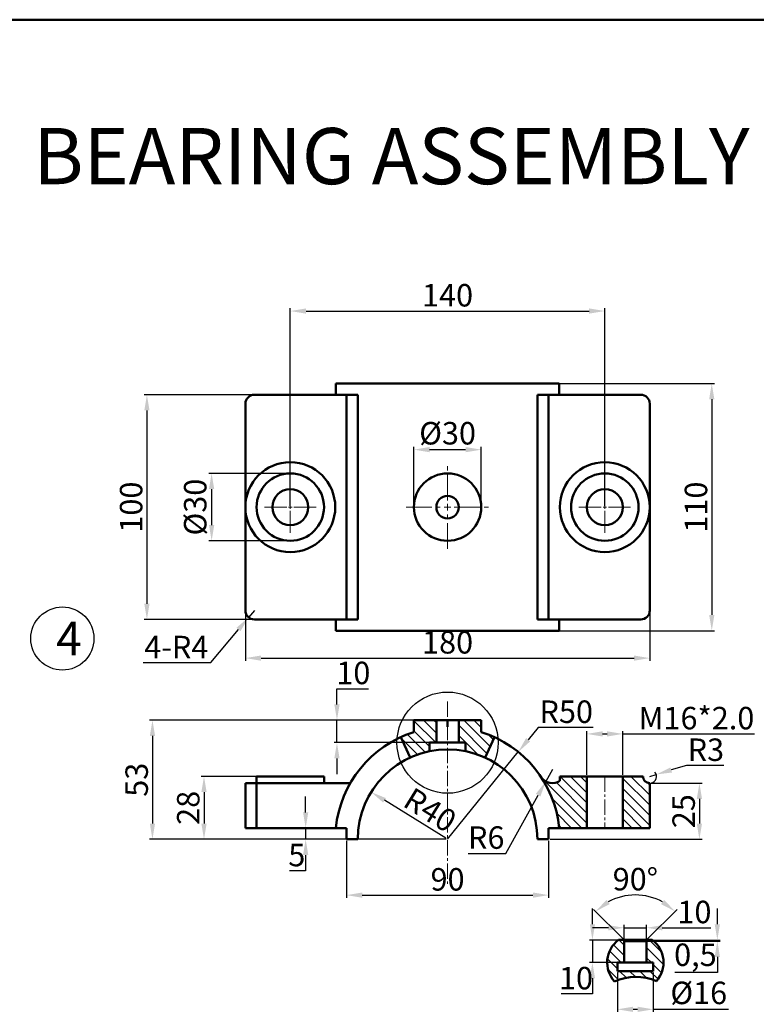
# Model space of a CAD drawing. Units: millimetres. Extents: x -68 to 1086, y -293 to 557.
# Tile 3 of 4: x 373 to 701, y 119 to 557. Entities that reach past the tile are written whole.
import ezdxf

# ---------------------------------------------------------------- set-up
doc = ezdxf.new("R2010")
doc.units = ezdxf.units.MM
doc.header["$LTSCALE"] = 0.6
doc.linetypes.add('CENTER2', pattern=[28.575, 19.05, -3.175, 3.175, -3.175])
for name, color, linetype, lineweight in [('M-CNTR', 1, 'CENTER2', 18), ('M-DIMS', 2, 'Continuous', 25), ('M-HATC', 8, 'Continuous', 18), ('M-OUTL', 7, 'Continuous', 50), ('M-SYMB', 4, 'Continuous', 25), ('M-TEXT', 3, 'Continuous', 25)]:
    doc.layers.add(name, color=color, linetype=linetype, lineweight=lineweight)
doc.styles.get("Standard").update_dxf_attribs({"font": 'arial.ttf'})
doc.dimstyles.new('ISO-25', dxfattribs={"dimtxt": 10, "dimasz": 7, "dimexe": 1.25, "dimexo": 0.625, "dimtad": 1, "dimtoh": 1, "dimtxsty": 'Standard', "dimcen": 2.5, "dimadec": 0, "dimazin": 0, "dimtfac": 1, "dimtmove": 0, "dimatfit": 3, "dimfxl": 1, "dimarcsym": 0})
pattern_1 = [(135, (-319.924, -184.7082), (-2.245064, -2.245064), [])]

# ---------------------------------------------------------------- blocks, each defined once
blk = doc.blocks.new('*U22')
at = {"layer": 'M-CNTR', "color": 0, "transparency": 16777216}
for p, q in [((0, 1.6), (0, 11.5)), ((-11.5, 0), (-1.6, 0)), ((1.6, 0), (11.5, 0)), ((0, -11.5), (0, -1.6))]:
    blk.add_line(p, q, dxfattribs=at)
at = {"layer": 'M-CNTR', "color": 0, "linetype": 'Continuous', "transparency": 16777216}
for p, q in [((-0.8, 0), (0.8, 0)), ((0, -0.8), (0, 0.8))]:
    blk.add_line(p, q, dxfattribs=at)
blk = doc.blocks.new('*U23')
at = {"layer": 'M-CNTR', "color": 0, "transparency": 16777216}
for p, q in [((0, 1.6), (0, 11.5)), ((-11.5, 0), (-1.6, 0)), ((1.6, 0), (11.5, 0)), ((0, -11.5), (0, -1.6))]:
    blk.add_line(p, q, dxfattribs=at)
at = {"layer": 'M-CNTR', "color": 0, "linetype": 'Continuous', "transparency": 16777216}
for p, q in [((-0.8, 0), (0.8, 0)), ((0, -0.8), (0, 0.8))]:
    blk.add_line(p, q, dxfattribs=at)
blk = doc.blocks.new('*U24')
at = {"layer": 'M-CNTR', "color": 0, "transparency": 16777216}
for p, q in [((0, 3), (0, 18.5)), ((-18.5, 0), (-3, 0)), ((3, 0), (18.5, 0)), ((0, -18.5), (0, -3))]:
    blk.add_line(p, q, dxfattribs=at)
at = {"layer": 'M-CNTR', "color": 0, "linetype": 'Continuous', "transparency": 16777216}
for p, q in [((-1.5, 0), (1.5, 0)), ((0, -1.5), (0, 1.5))]:
    blk.add_line(p, q, dxfattribs=at)
blk = doc.blocks.new('*D25')
at = {"layer": 'Defpoints', "color": 0, "ltscale": 0.6, "transparency": 16777216}
for p in [(563.31, 244.93), (431.94, 191.93), (563.31, 191.93)]:
    blk.add_point(p, dxfattribs=at)
at = {"layer": 'M-DIMS', "color": 0, "lineweight": -2, "ltscale": 0.6, "transparency": 16777216}
for p, q in [((562.68, 244.93), (430.69, 244.93)), ((431.94, 237.93), (431.94, 198.93)), ((562.68, 191.93), (430.69, 191.93))]:
    blk.add_line(p, q, dxfattribs=at)
at = {"layer": 'M-DIMS', "color": 0, "ltscale": 0.6, "transparency": 16777216}
for points in [[(430.78, 237.93), (433.11, 237.93), (431.94, 244.93)], [(430.78, 198.93), (433.11, 198.93), (431.94, 191.93)]]:
    blk.add_solid(points, dxfattribs=at)
at = {"layer": 'M-DIMS', "color": 0, "ltscale": 0.6, "transparency": 16777216, "insert": (426.21, 218.43), "char_height": 10, "attachment_point": 5, "rotation": 90}
blk.add_mtext('53', dxfattribs=at)
blk = doc.blocks.new('*D26')
at = {"layer": 'Defpoints', "color": 0, "ltscale": 0.6, "transparency": 16777216}
for p in [(493.31, 219.93), (454.89, 191.93), (493.31, 191.93)]:
    blk.add_point(p, dxfattribs=at)
at = {"layer": 'M-DIMS', "color": 0, "lineweight": -2, "ltscale": 0.6, "transparency": 16777216}
for p, q in [((492.68, 219.93), (453.64, 219.93)), ((454.89, 212.93), (454.89, 198.93)), ((492.68, 191.93), (453.64, 191.93))]:
    blk.add_line(p, q, dxfattribs=at)
at = {"layer": 'M-DIMS', "color": 0, "ltscale": 0.6, "transparency": 16777216}
for points in [[(453.72, 212.93), (456.05, 212.93), (454.89, 219.93)], [(453.72, 198.93), (456.05, 198.93), (454.89, 191.93)]]:
    blk.add_solid(points, dxfattribs=at)
at = {"layer": 'M-DIMS', "color": 0, "ltscale": 0.6, "transparency": 16777216, "insert": (449.16, 205.93), "char_height": 10, "attachment_point": 5, "rotation": 90}
blk.add_mtext('28', dxfattribs=at)
blk = doc.blocks.new('*D27')
at = {"layer": 'Defpoints', "color": 0, "ltscale": 0.6, "transparency": 16777216}
for p in [(563.31, 244.93), (514.07, 234.93), (563.31, 234.93)]:
    blk.add_point(p, dxfattribs=at)
at = {"layer": 'M-DIMS', "color": 0, "lineweight": -2, "ltscale": 0.6, "transparency": 16777216}
for p, q in [((514.07, 251.93), (514.07, 258.93)), ((514.07, 258.93), (528.04, 258.93)), ((562.68, 244.93), (512.82, 244.93)), ((514.07, 234.93), (514.07, 244.93)), ((562.68, 234.93), (512.82, 234.93)), ((514.07, 227.93), (514.07, 220.93))]:
    blk.add_line(p, q, dxfattribs=at)
at = {"layer": 'M-DIMS', "color": 0, "ltscale": 0.6, "transparency": 16777216}
for points in [[(512.9, 251.93), (515.24, 251.93), (514.07, 244.93)], [(512.9, 227.93), (515.24, 227.93), (514.07, 234.93)]]:
    blk.add_solid(points, dxfattribs=at)
at = {"layer": 'M-DIMS', "color": 0, "ltscale": 0.6, "transparency": 16777216, "insert": (521.37, 264.66), "char_height": 10, "attachment_point": 5}
blk.add_mtext('10', dxfattribs=at)
blk = doc.blocks.new('*D28')
at = {"layer": 'Defpoints', "color": 0, "ltscale": 0.6, "transparency": 16777216}
for p in [(653.31, 216.93), (608.31, 191.93), (675.42, 191.93)]:
    blk.add_point(p, dxfattribs=at)
at = {"layer": 'M-DIMS', "color": 0, "lineweight": -2, "ltscale": 0.6, "transparency": 16777216}
for p, q in [((653.93, 216.93), (676.67, 216.93)), ((675.42, 209.93), (675.42, 198.93)), ((608.93, 191.93), (676.67, 191.93))]:
    blk.add_line(p, q, dxfattribs=at)
at = {"layer": 'M-DIMS', "color": 0, "ltscale": 0.6, "transparency": 16777216}
for points in [[(674.25, 209.93), (676.58, 209.93), (675.42, 216.93)], [(674.25, 198.93), (676.58, 198.93), (675.42, 191.93)]]:
    blk.add_solid(points, dxfattribs=at)
at = {"layer": 'M-DIMS', "color": 0, "ltscale": 0.6, "transparency": 16777216, "insert": (669.69, 204.43), "char_height": 10, "attachment_point": 5, "rotation": 90}
blk.add_mtext('25', dxfattribs=at)
blk = doc.blocks.new('*D29')
at = {"layer": 'Defpoints', "color": 0, "ltscale": 0.6, "transparency": 16777216}
for p in [(518.31, 191.93), (608.31, 191.93), (608.31, 167.1)]:
    blk.add_point(p, dxfattribs=at)
at = {"layer": 'M-DIMS', "color": 0, "lineweight": -2, "ltscale": 0.6, "transparency": 16777216}
for p, q in [((518.31, 191.31), (518.31, 165.85)), ((608.31, 191.31), (608.31, 165.85)), ((525.31, 167.1), (601.31, 167.1))]:
    blk.add_line(p, q, dxfattribs=at)
at = {"layer": 'M-DIMS', "color": 0, "ltscale": 0.6, "transparency": 16777216}
for points in [[(525.31, 168.26), (525.31, 165.93), (518.31, 167.1)], [(601.31, 168.26), (601.31, 165.93), (608.31, 167.1)]]:
    blk.add_solid(points, dxfattribs=at)
at = {"layer": 'M-DIMS', "color": 0, "ltscale": 0.6, "transparency": 16777216, "insert": (563.31, 172.83), "char_height": 10, "attachment_point": 5}
blk.add_mtext('90', dxfattribs=at)
blk = doc.blocks.new('*D30')
at = {"layer": 'Defpoints', "color": 0, "ltscale": 0.6, "transparency": 16777216}
for p in [(529.28, 212.96), (563.31, 191.93)]:
    blk.add_point(p, dxfattribs=at)
at = {"layer": 'M-DIMS', "color": 0, "lineweight": -2, "ltscale": 0.6, "transparency": 16777216}
blk.add_line((562.55, 192.4), (535.24, 209.28), dxfattribs=at)
at = {"layer": 'M-DIMS', "color": 0, "ltscale": 0.6, "transparency": 16777216}
blk.add_solid([(535.85, 210.27), (534.63, 208.29), (529.28, 212.96)], dxfattribs=at)
at = {"layer": 'M-DIMS', "color": 0, "ltscale": 0.6, "transparency": 16777216, "insert": (554.89, 203.88), "char_height": 10, "attachment_point": 5, "rotation": 328.282}
blk.add_mtext('R40', dxfattribs=at)
blk = doc.blocks.new('*D31')
at = {"layer": 'Defpoints', "color": 0, "ltscale": 0.6, "transparency": 16777216}
for p in [(594.77, 230.8), (563.31, 191.93)]:
    blk.add_point(p, dxfattribs=at)
at = {"layer": 'M-DIMS', "color": 0, "lineweight": -2, "ltscale": 0.6, "transparency": 16777216}
for p, q in [((603.58, 241.68), (599.17, 236.24)), ((628.06, 241.68), (603.58, 241.68)), ((563.31, 191.93), (594.77, 230.8))]:
    blk.add_line(p, q, dxfattribs=at)
at = {"layer": 'M-DIMS', "color": 0, "ltscale": 0.6, "transparency": 16777216}
blk.add_solid([(598.26, 236.97), (600.08, 235.5), (594.77, 230.8)], dxfattribs=at)
at = {"layer": 'M-DIMS', "color": 0, "ltscale": 0.6, "transparency": 16777216, "insert": (616.13, 247.41), "char_height": 10, "attachment_point": 5}
blk.add_mtext('R50', dxfattribs=at)
blk = doc.blocks.new('*D32')
at = {"layer": 'Defpoints', "color": 0, "ltscale": 0.6, "transparency": 16777216}
for p in [(609.95, 222.93), (607.03, 217.69)]:
    blk.add_point(p, dxfattribs=at)
at = {"layer": 'M-DIMS', "color": 0, "lineweight": -2, "ltscale": 0.6, "transparency": 16777216}
for p, q in [((609.95, 222.93), (607.03, 217.69)), ((589.2, 185.68), (603.62, 211.57)), ((572.46, 185.68), (589.2, 185.68))]:
    blk.add_line(p, q, dxfattribs=at)
at = {"layer": 'M-DIMS', "color": 0, "ltscale": 0.6, "transparency": 16777216}
blk.add_solid([(602.6, 212.14), (604.64, 211.01), (607.03, 217.69)], dxfattribs=at)
at = {"layer": 'M-DIMS', "color": 0, "ltscale": 0.6, "transparency": 16777216, "insert": (580.52, 191.41), "char_height": 10, "attachment_point": 5}
blk.add_mtext('R6', dxfattribs=at)
blk = doc.blocks.new('*D33')
at = {"layer": 'Defpoints', "color": 0, "ltscale": 0.6, "transparency": 16777216}
for p in [(518.31, 196.93), (500.14, 191.93), (518.31, 191.93)]:
    blk.add_point(p, dxfattribs=at)
at = {"layer": 'M-DIMS', "color": 0, "lineweight": -2, "ltscale": 0.6, "transparency": 16777216}
for p, q in [((500.14, 203.93), (500.14, 210.93)), ((517.68, 196.93), (498.89, 196.93)), ((500.14, 196.93), (500.14, 191.93)), ((517.68, 191.93), (498.89, 191.93)), ((500.14, 184.93), (500.14, 177.93)), ((500.14, 177.93), (492.88, 177.93))]:
    blk.add_line(p, q, dxfattribs=at)
at = {"layer": 'M-DIMS', "color": 0, "ltscale": 0.6, "transparency": 16777216}
for points in [[(498.97, 203.93), (501.3, 203.93), (500.14, 196.93)], [(498.97, 184.93), (501.3, 184.93), (500.14, 191.93)]]:
    blk.add_solid(points, dxfattribs=at)
at = {"layer": 'M-DIMS', "color": 0, "ltscale": 0.6, "transparency": 16777216, "insert": (496.2, 183.64), "char_height": 10, "attachment_point": 5}
blk.add_mtext('5', dxfattribs=at)
blk = doc.blocks.new('*D34')
at = {"layer": 'Defpoints', "color": 0, "ltscale": 0.6, "transparency": 16777216}
for p in [(638.9, 133.33), (654.9, 133.33), (654.9, 116.29)]:
    blk.add_point(p, dxfattribs=at)
at = {"layer": 'M-DIMS', "color": 0, "lineweight": -2, "ltscale": 0.6, "transparency": 16777216}
for p, q in [((638.9, 132.7), (638.9, 115.04)), ((654.9, 132.7), (654.9, 115.04)), ((645.9, 116.29), (647.9, 116.29)), ((654.9, 116.29), (688.35, 116.29))]:
    blk.add_line(p, q, dxfattribs=at)
at = {"layer": 'M-DIMS', "color": 0, "ltscale": 0.6, "transparency": 16777216}
for points in [[(645.9, 117.46), (645.9, 115.12), (638.9, 116.29)], [(647.9, 117.46), (647.9, 115.12), (654.9, 116.29)]]:
    blk.add_solid(points, dxfattribs=at)
at = {"layer": 'M-DIMS', "color": 0, "ltscale": 0.6, "transparency": 16777216, "insert": (675.12, 122.3), "char_height": 10, "attachment_point": 5}
blk.add_mtext('%%C16', dxfattribs=at)
blk = doc.blocks.new('*D35')
at = {"layer": 'Defpoints', "color": 0, "ltscale": 0.6, "transparency": 16777216}
for p in [(641.9, 147.13), (627.79, 137.13), (641.9, 137.13)]:
    blk.add_point(p, dxfattribs=at)
at = {"layer": 'M-DIMS', "color": 0, "lineweight": -2, "ltscale": 0.6, "transparency": 16777216}
for p, q in [((627.79, 154.13), (627.79, 161.13)), ((641.28, 147.13), (626.54, 147.13)), ((627.79, 147.13), (627.79, 137.13)), ((641.28, 137.13), (626.54, 137.13)), ((627.79, 130.13), (627.79, 123.13)), ((627.79, 123.13), (613.82, 123.13))]:
    blk.add_line(p, q, dxfattribs=at)
at = {"layer": 'M-DIMS', "color": 0, "ltscale": 0.6, "transparency": 16777216}
for points in [[(626.63, 154.13), (628.96, 154.13), (627.79, 147.13)], [(626.63, 130.13), (628.96, 130.13), (627.79, 137.13)]]:
    blk.add_solid(points, dxfattribs=at)
at = {"layer": 'M-DIMS', "color": 0, "ltscale": 0.6, "transparency": 16777216, "insert": (620.49, 128.87), "char_height": 10, "attachment_point": 5}
blk.add_mtext('10', dxfattribs=at)
blk = doc.blocks.new('*D36')
at = {"layer": 'Defpoints', "color": 0, "ltscale": 0.6, "transparency": 16777216}
for p in [(653.38, 166.33), (641.9, 147.13), (642.4, 146.63), (651.4, 146.63), (651.9, 147.13)]:
    blk.add_point(p, dxfattribs=at)
at = {"layer": 'M-DIMS', "color": 0, "lineweight": -2, "ltscale": 0.6, "transparency": 16777216}
for p, q in [((641.46, 147.58), (628.31, 160.73)), ((652.34, 147.58), (665.49, 160.73))]:
    blk.add_line(p, q, dxfattribs=at)
blk.add_arc((646.9, 142.13), 25.05, 61.0658, 118.9342, dxfattribs=at)
at = {"layer": 'M-DIMS', "color": 0, "ltscale": 0.6, "transparency": 16777216}
for points in [[(635.48, 163.12), (634.08, 164.99), (629.19, 159.85)], [(659.72, 164.99), (658.32, 163.12), (664.61, 159.85)]]:
    blk.add_solid(points, dxfattribs=at)
at = {"layer": 'M-DIMS', "color": 0, "ltscale": 0.6, "transparency": 16777216, "insert": (646.9, 172.91), "char_height": 10, "attachment_point": 5}
blk.add_mtext('90°', dxfattribs=at)
blk = doc.blocks.new('*D37')
at = {"layer": 'Defpoints', "color": 0, "ltscale": 0.6, "transparency": 16777216}
for p in [(651.9, 152.57), (641.9, 147.13), (651.9, 147.13)]:
    blk.add_point(p, dxfattribs=at)
at = {"layer": 'M-DIMS', "color": 0, "lineweight": -2, "ltscale": 0.6, "transparency": 16777216}
for p, q in [((641.9, 147.76), (641.9, 153.82)), ((651.9, 147.76), (651.9, 153.82)), ((634.9, 152.57), (627.9, 152.57)), ((641.9, 152.57), (651.9, 152.57)), ((658.9, 152.57), (680.5, 152.57))]:
    blk.add_line(p, q, dxfattribs=at)
at = {"layer": 'M-DIMS', "color": 0, "ltscale": 0.6, "transparency": 16777216}
for points in [[(634.9, 153.74), (634.9, 151.41), (641.9, 152.57)], [(658.9, 153.74), (658.9, 151.41), (651.9, 152.57)]]:
    blk.add_solid(points, dxfattribs=at)
at = {"layer": 'M-DIMS', "color": 0, "ltscale": 0.6, "transparency": 16777216, "insert": (673.2, 158.3), "char_height": 10, "attachment_point": 5}
blk.add_mtext('10', dxfattribs=at)
blk = doc.blocks.new('*D38')
at = {"layer": 'Defpoints', "color": 0, "ltscale": 0.6, "transparency": 16777216}
for p in [(651.29, 147.13), (651.29, 146.63), (683.4, 146.63)]:
    blk.add_point(p, dxfattribs=at)
at = {"layer": 'M-DIMS', "color": 0, "lineweight": -2, "ltscale": 0.6, "transparency": 16777216}
for p, q in [((683.4, 154.13), (683.4, 161.13)), ((651.92, 147.13), (684.65, 147.13)), ((651.92, 146.63), (684.65, 146.63)), ((683.4, 147.13), (683.4, 146.63)), ((683.4, 139.63), (683.4, 132.63)), ((683.4, 132.63), (664.49, 132.63))]:
    blk.add_line(p, q, dxfattribs=at)
at = {"layer": 'M-DIMS', "color": 0, "ltscale": 0.6, "transparency": 16777216}
for points in [[(682.23, 154.13), (684.57, 154.13), (683.4, 147.13)], [(682.23, 139.63), (684.57, 139.63), (683.4, 146.63)]]:
    blk.add_solid(points, dxfattribs=at)
at = {"layer": 'M-DIMS', "color": 0, "ltscale": 0.6, "transparency": 16777216, "insert": (673.63, 139.27), "char_height": 10, "attachment_point": 5}
blk.add_mtext('0,5', dxfattribs=at)
blk = doc.blocks.new('*D39')
at = {"layer": 'Defpoints', "color": 0, "ltscale": 0.6, "transparency": 16777216}
for p in [(633.31, 426.96), (493.31, 339.73), (633.31, 339.73)]:
    blk.add_point(p, dxfattribs=at)
at = {"layer": 'M-DIMS', "color": 0, "lineweight": -2, "ltscale": 0.6, "transparency": 16777216}
for p, q in [((493.31, 340.35), (493.31, 428.21)), ((500.31, 426.96), (626.31, 426.96)), ((633.31, 340.35), (633.31, 428.21))]:
    blk.add_line(p, q, dxfattribs=at)
at = {"layer": 'M-DIMS', "color": 0, "ltscale": 0.6, "transparency": 16777216}
for points in [[(500.31, 428.13), (500.31, 425.8), (493.31, 426.96)], [(626.31, 428.13), (626.31, 425.8), (633.31, 426.96)]]:
    blk.add_solid(points, dxfattribs=at)
at = {"layer": 'M-DIMS', "color": 0, "ltscale": 0.6, "transparency": 16777216, "insert": (563.31, 432.69), "char_height": 10, "attachment_point": 5}
blk.add_mtext('140', dxfattribs=at)
blk = doc.blocks.new('*D40')
at = {"layer": 'Defpoints', "color": 0, "ltscale": 0.6, "transparency": 16777216}
for p in [(483.88, 389.73), (429.47, 289.73), (483.88, 289.73)]:
    blk.add_point(p, dxfattribs=at)
at = {"layer": 'M-DIMS', "color": 0, "lineweight": -2, "ltscale": 0.6, "transparency": 16777216}
for p, q in [((483.25, 389.73), (428.22, 389.73)), ((429.47, 382.73), (429.47, 296.73)), ((483.25, 289.73), (428.22, 289.73))]:
    blk.add_line(p, q, dxfattribs=at)
at = {"layer": 'M-DIMS', "color": 0, "ltscale": 0.6, "transparency": 16777216}
for points in [[(428.31, 382.73), (430.64, 382.73), (429.47, 389.73)], [(428.31, 296.73), (430.64, 296.73), (429.47, 289.73)]]:
    blk.add_solid(points, dxfattribs=at)
at = {"layer": 'M-DIMS', "color": 0, "ltscale": 0.6, "transparency": 16777216, "insert": (423.74, 339.73), "char_height": 10, "attachment_point": 5, "rotation": 90}
blk.add_mtext('100', dxfattribs=at)
blk = doc.blocks.new('*D41')
at = {"layer": 'Defpoints', "color": 0, "ltscale": 0.6, "transparency": 16777216}
for p in [(493.31, 354.73), (458.28, 324.73), (493.31, 324.73)]:
    blk.add_point(p, dxfattribs=at)
at = {"layer": 'M-DIMS', "color": 0, "lineweight": -2, "ltscale": 0.6, "transparency": 16777216}
for p, q in [((492.68, 354.73), (457.03, 354.73)), ((458.28, 347.73), (458.28, 331.73)), ((492.68, 324.73), (457.03, 324.73))]:
    blk.add_line(p, q, dxfattribs=at)
at = {"layer": 'M-DIMS', "color": 0, "ltscale": 0.6, "transparency": 16777216}
for points in [[(457.11, 347.73), (459.45, 347.73), (458.28, 354.73)], [(457.11, 331.73), (459.45, 331.73), (458.28, 324.73)]]:
    blk.add_solid(points, dxfattribs=at)
at = {"layer": 'M-DIMS', "color": 0, "ltscale": 0.6, "transparency": 16777216, "insert": (452.27, 339.73), "char_height": 10, "attachment_point": 5, "rotation": 90}
blk.add_mtext('%%C30', dxfattribs=at)
blk = doc.blocks.new('*D42')
at = {"layer": 'Defpoints', "color": 0, "ltscale": 0.6, "transparency": 16777216}
for p in [(477.31, 293.73), (474.74, 290.66)]:
    blk.add_point(p, dxfattribs=at)
at = {"layer": 'M-DIMS', "color": 0, "lineweight": -2, "ltscale": 0.6, "transparency": 16777216}
for p, q in [((477.31, 293.73), (474.74, 290.66)), ((457.9, 270.55), (470.25, 285.29)), ((427.85, 270.55), (457.9, 270.55))]:
    blk.add_line(p, q, dxfattribs=at)
at = {"layer": 'M-DIMS', "color": 0, "ltscale": 0.6, "transparency": 16777216}
blk.add_solid([(469.35, 286.04), (471.14, 284.54), (474.74, 290.66)], dxfattribs=at)
at = {"layer": 'M-DIMS', "color": 0, "ltscale": 0.6, "transparency": 16777216, "insert": (442.56, 276.18), "char_height": 10, "attachment_point": 5}
blk.add_mtext('4-R4', dxfattribs=at)
blk = doc.blocks.new('*D43')
at = {"layer": 'Defpoints', "color": 0, "ltscale": 0.6, "transparency": 16777216}
for p in [(473.31, 306.54), (653.31, 306.54), (653.31, 272.55)]:
    blk.add_point(p, dxfattribs=at)
at = {"layer": 'M-DIMS', "color": 0, "lineweight": -2, "ltscale": 0.6, "transparency": 16777216}
for p, q in [((473.31, 305.91), (473.31, 271.3)), ((653.31, 305.91), (653.31, 271.3)), ((480.31, 272.55), (646.31, 272.55))]:
    blk.add_line(p, q, dxfattribs=at)
at = {"layer": 'M-DIMS', "color": 0, "ltscale": 0.6, "transparency": 16777216}
for points in [[(480.31, 273.72), (480.31, 271.38), (473.31, 272.55)], [(646.31, 273.72), (646.31, 271.38), (653.31, 272.55)]]:
    blk.add_solid(points, dxfattribs=at)
at = {"layer": 'M-DIMS', "color": 0, "ltscale": 0.6, "transparency": 16777216, "insert": (563.31, 278.28), "char_height": 10, "attachment_point": 5}
blk.add_mtext('180', dxfattribs=at)
blk = doc.blocks.new('*D44')
at = {"layer": 'Defpoints', "color": 0, "ltscale": 0.6, "transparency": 16777216}
for p in [(586.76, 394.73), (586.76, 284.73), (680.92, 284.73)]:
    blk.add_point(p, dxfattribs=at)
at = {"layer": 'M-DIMS', "color": 0, "lineweight": -2, "ltscale": 0.6, "transparency": 16777216}
for p, q in [((587.39, 394.73), (682.17, 394.73)), ((680.92, 387.73), (680.92, 291.73)), ((587.39, 284.73), (682.17, 284.73))]:
    blk.add_line(p, q, dxfattribs=at)
at = {"layer": 'M-DIMS', "color": 0, "ltscale": 0.6, "transparency": 16777216}
for points in [[(679.76, 387.73), (682.09, 387.73), (680.92, 394.73)], [(679.76, 291.73), (682.09, 291.73), (680.92, 284.73)]]:
    blk.add_solid(points, dxfattribs=at)
at = {"layer": 'M-DIMS', "color": 0, "ltscale": 0.6, "transparency": 16777216, "insert": (675.19, 339.73), "char_height": 10, "attachment_point": 5, "rotation": 90}
blk.add_mtext('110', dxfattribs=at)
blk = doc.blocks.new('*D45')
at = {"layer": 'Defpoints', "color": 0, "ltscale": 0.6, "transparency": 16777216}
for p in [(578.31, 365.29), (548.31, 339.73), (578.31, 339.73)]:
    blk.add_point(p, dxfattribs=at)
at = {"layer": 'M-DIMS', "color": 0, "lineweight": -2, "ltscale": 0.6, "transparency": 16777216}
for p, q in [((548.31, 340.35), (548.31, 366.54)), ((555.31, 365.29), (571.31, 365.29)), ((578.31, 340.35), (578.31, 366.54))]:
    blk.add_line(p, q, dxfattribs=at)
at = {"layer": 'M-DIMS', "color": 0, "ltscale": 0.6, "transparency": 16777216}
for points in [[(555.31, 366.46), (555.31, 364.13), (548.31, 365.29)], [(571.31, 366.46), (571.31, 364.13), (578.31, 365.29)]]:
    blk.add_solid(points, dxfattribs=at)
at = {"layer": 'M-DIMS', "color": 0, "ltscale": 0.6, "transparency": 16777216, "insert": (563.31, 371.3), "char_height": 10, "attachment_point": 5}
blk.add_mtext('%%C30', dxfattribs=at)
blk = doc.blocks.new('*D46')
at = {"layer": 'Defpoints', "color": 0, "ltscale": 0.6, "transparency": 16777216}
for p in [(641.31, 238.83), (625.31, 219.93), (641.31, 219.93)]:
    blk.add_point(p, dxfattribs=at)
at = {"layer": 'M-DIMS', "color": 0, "lineweight": -2, "ltscale": 0.6, "transparency": 16777216}
for p, q in [((625.31, 220.56), (625.31, 240.08)), ((632.31, 238.83), (634.31, 238.83)), ((641.31, 220.56), (641.31, 240.08)), ((641.31, 238.83), (699.89, 238.83))]:
    blk.add_line(p, q, dxfattribs=at)
at = {"layer": 'M-DIMS', "color": 0, "ltscale": 0.6, "transparency": 16777216}
for points in [[(632.31, 240), (632.31, 237.66), (625.31, 238.83)], [(634.31, 240), (634.31, 237.66), (641.31, 238.83)]]:
    blk.add_solid(points, dxfattribs=at)
at = {"layer": 'M-DIMS', "color": 0, "ltscale": 0.6, "transparency": 16777216, "insert": (674.1, 244.56), "char_height": 10, "attachment_point": 5}
blk.add_mtext('M16*2.0', dxfattribs=at)
blk = doc.blocks.new('*D47')
at = {"layer": 'Defpoints', "color": 0, "ltscale": 0.6, "transparency": 16777216}
for p in [(653.31, 219.93), (656.19, 220.78)]:
    blk.add_point(p, dxfattribs=at)
at = {"layer": 'M-DIMS', "color": 0, "lineweight": -2, "ltscale": 0.6, "transparency": 16777216}
for p, q in [((669.61, 224.76), (662.9, 222.77)), ((686.36, 224.76), (669.61, 224.76)), ((653.31, 219.93), (656.19, 220.78))]:
    blk.add_line(p, q, dxfattribs=at)
blk.add_arc((653.31, 219.93), 3, 281.9366, 40.3615, dxfattribs=at)
at = {"layer": 'M-DIMS', "color": 0, "ltscale": 0.6, "transparency": 16777216}
blk.add_solid([(662.57, 223.89), (663.23, 221.65), (656.19, 220.78)], dxfattribs=at)
at = {"layer": 'M-DIMS', "color": 0, "ltscale": 0.6, "transparency": 16777216, "insert": (678.3, 230.49), "char_height": 10, "attachment_point": 5}
blk.add_mtext('R3', dxfattribs=at)

msp = doc.modelspace()

# ---------------------------------------------------------------- hatches: boundary and pattern name
at = {"layer": 'M-HATC', "ltscale": 0.6}
h = msp.add_hatch(dxfattribs=at)
h.set_pattern_fill('ANSI31', color=256, angle=90)
h.set_pattern_definition(pattern_1)
h.paths.add_polyline_path([(578.31, 239.629), (578.31, 244.932), (568.31, 244.932), (568.31, 234.932), (571.31, 234.932), (571.31, 231.124, -0.0573623), (580.005, 228.281), (584.179, 237.369, 0.0314762)])
h.paths.add_polyline_path([(548.31, 239.629, 0.0314762), (542.441, 237.369), (546.615, 228.281, -0.0573623), (555.31, 231.124), (555.31, 234.932), (558.31, 234.932), (558.31, 244.932), (548.31, 244.932)])
h = msp.add_hatch(dxfattribs=at)
h.set_pattern_fill('ANSI31', color=256, angle=90)
h.set_pattern_definition(pattern_1)
h.paths.add_polyline_path([(641.31, 196.932), (653.31, 196.932), (653.31, 216.932, -0.4142136), (650.31, 219.932), (641.31, 219.932)])
h.paths.add_polyline_path([(625.31, 219.932), (613.31, 219.932), (613.31, 217.963, -0.4166654), (604.95, 219.61, -0.122223), (613.059, 196.932), (625.31, 196.932)])
h = msp.add_hatch(dxfattribs=at)
h.set_pattern_fill('ANSI31', color=256, angle=90)
h.set_pattern_definition([(135, (-327.175, -197.2673), (-2.245064, -2.245064), [])])
h.paths.add_polyline_path([(641.9, 147.135), (639.343, 147.135, 0.4410804), (637.627, 128.702, -0.2037605), (656.323, 128.869, 0.4357373), (654.457, 147.135), (651.9, 147.135), (651.9, 137.135), (654.9, 137.135), (654.9, 133.327), (638.9, 133.327), (638.9, 137.135), (641.9, 137.135)])

# ---------------------------------------------------------------- linework, layer by layer
at = {"layer": 'M-CNTR', "ltscale": 0.6}
for p, q in [((563.31, 253.239), (563.31, 171.001)), ((633.31, 219.932), (633.31, 196.932))]:
    msp.add_line(p, q, dxfattribs=at)
at = {"layer": 'M-OUTL', "ltscale": 0.6}
for p, q in [((513.561, 394.727), (613.059, 394.727)), ((513.561, 394.727), (513.561, 389.727)), ((613.059, 394.727), (613.059, 389.727)), ((473.31, 293.727), (473.31, 385.727)), ((477.31, 389.727), (513.561, 389.727)), ((513.561, 389.727), (523.31, 389.727)), ((518.31, 389.727), (518.31, 289.727)), ((523.31, 389.727), (523.31, 289.727)), ((603.31, 389.727), (603.31, 289.727)), ((603.31, 389.727), (649.31, 389.727)), ((608.31, 389.727), (608.31, 289.727)), ((653.31, 385.727), (653.31, 293.727)), ((477.31, 289.727), (513.561, 289.727)), ((513.561, 289.727), (523.31, 289.727)), ((513.561, 289.727), (513.561, 284.727)), ((603.31, 289.727), (649.31, 289.727)), ((613.059, 289.727), (613.059, 284.727)), ((613.059, 284.727), (513.561, 284.727)), ((548.31, 244.932), (578.31, 244.932)), ((548.31, 244.932), (548.31, 239.629)), ((558.31, 244.932), (568.31, 244.932)), ((558.31, 234.932), (558.31, 244.932)), ((563.31, 244.932), (563.31, 241.932)), ((568.31, 244.932), (568.31, 234.932)), ((578.31, 244.932), (578.31, 239.629)), ((542.441, 237.369), (546.615, 228.281)), ((584.179, 237.369), (580.005, 228.281)), ((555.31, 231.124), (555.31, 234.932)), ((555.31, 234.932), (558.31, 234.932)), ((568.31, 234.932), (558.31, 234.932)), ((568.31, 234.932), (571.31, 234.932)), ((571.31, 234.932), (571.31, 231.124)), ((508.31, 219.932), (478.31, 219.932)), ((478.31, 219.932), (478.31, 196.932)), ((508.31, 219.932), (508.31, 216.932)), ((613.31, 219.932), (650.31, 219.932)), ((613.31, 219.932), (613.31, 217.963)), ((625.31, 219.932), (625.31, 196.932)), ((641.31, 219.932), (641.31, 196.932)), ((473.31, 216.932), (520.009, 216.932)), ((473.31, 216.932), (473.31, 196.932)), ((653.31, 216.932), (653.31, 196.932)), ((513.561, 196.932), (473.31, 196.932)), ((518.31, 196.932), (513.561, 196.932)), ((518.31, 196.932), (518.31, 191.932)), ((653.31, 196.932), (608.31, 196.932)), ((608.31, 196.932), (608.31, 191.932)), ((523.31, 191.932), (518.31, 191.932)), ((608.31, 191.932), (603.31, 191.932)), ((641.9, 147.135), (639.343, 147.135)), ((641.9, 147.135), (651.9, 147.135)), ((641.9, 147.135), (641.9, 147.135)), ((642.4, 146.635), (641.9, 147.135)), ((641.9, 147.135), (641.9, 137.135)), ((641.9, 146.635), (651.9, 146.635)), ((651.4, 146.635), (651.9, 147.135)), ((651.9, 147.135), (651.9, 147.135)), ((651.9, 147.135), (651.9, 137.135)), ((651.9, 147.135), (654.457, 147.135)), ((638.9, 133.327), (638.9, 137.135)), ((641.9, 137.135), (638.9, 137.135)), ((651.9, 137.135), (641.9, 137.135)), ((651.9, 137.135), (654.9, 137.135)), ((654.9, 137.135), (654.9, 133.327)), ((638.9, 133.327), (654.9, 133.327))]:
    msp.add_line(p, q, dxfattribs=at)
msp.add_lwpolyline([(-68.392, 556.589), (1085.677, 556.589), (1085.677, -292.72), (-68.392, -292.72)], close=True, dxfattribs=at)
for centre, radius in [((493.31, 339.727), 20), ((633.31, 339.727), 20), ((493.31, 339.727), 15), ((563.31, 339.727), 15), ((633.31, 339.727), 15), ((493.31, 339.727), 8), ((633.31, 339.727), 8), ((563.31, 339.727), 5)]:
    msp.add_circle(centre, radius, dxfattribs=at)
for centre, radius, start, end in [((477.31, 385.727), 4, 90, 180), ((649.31, 385.727), 4, 0, 90), ((477.31, 293.727), 4, 180, 270), ((649.31, 293.727), 4, 270, 0), ((563.31, 191.932), 50, 107.4576, 174.26083), ((563.31, 191.932), 50, 5.73917, 72.5424), ((563.31, 191.932), 40, 0, 180), ((609.947, 222.932), 6, 213.61237, 304.09159), ((653.31, 219.932), 3, 180, 270), ((646.9, 137.135), 12.534, 127.0782, 222.28355), ((646.9, 137.135), 12.534, 318.74359, 52.9218), ((647.172, 106.799), 23.892, 67.47966, 113.54748)]:
    msp.add_arc(centre, radius, start, end, dxfattribs=at)
at = {"layer": 'M-SYMB', "ltscale": 0.6}
for centre, radius in [((391.851, 281.258), 14.053), ((563.31, 234.932), 22.515)]:
    msp.add_circle(centre, radius, dxfattribs=at)

# ---------------------------------------------------------------- block references
at = {"layer": 'M-CNTR'}
for name, p in [('*U24', (563.31, 339.727)), ('*U22', (493.31, 339.727)), ('*U23', (633.31, 339.727))]:
    msp.add_blockref(name, p, dxfattribs=at)

# ---------------------------------------------------------------- texts
at = {"layer": 'M-TEXT', "ltscale": 0.6, "attachment_point": 1}
for s, width, insert, char_height in [('BEARING ASSEMBLY', 392.3105, (378.882, 508.403), 25), ('4', 27.55708, (389.088, 288.789), 15)]:
    msp.add_mtext_dynamic_manual_height_columns(s, width=width, gutter_width=12.5, heights=[0], dxfattribs=dict(at, insert=insert, char_height=char_height))

# ---------------------------------------------------------------- dimensions: what is measured, and where the dimension line sits
at = {"layer": 'M-DIMS', "ltscale": 0.6}
for base, p1, p2, picture, middle in [((633.31, 426.962), (493.31, 339.727), (633.31, 339.727), '*D39', (563.31, 432.693)), ((653.31, 272.55), (473.31, 306.539), (653.31, 306.539), '*D43', (563.31, 278.28)), ((608.31, 167.098), (518.31, 191.932), (608.31, 191.932), '*D29', (563.31, 172.828)), ((651.9, 152.573), (641.9, 147.135), (651.9, 147.135), '*D37', (673.2, 158.303))]:
    dim = msp.add_linear_dim(base=base, p1=p1, p2=p2, dimstyle='ISO-25', override={"dimclrd": 0, "dimclre": 0, "dimclrt": 0}, dxfattribs=at)
    dim.commit()
    dim.dimension.update_dxf_attribs({"geometry": picture, "text_midpoint": middle})
for base, p1, p2, picture, middle in [((680.922, 284.727), (586.76, 394.727), (586.76, 284.727), '*D44', (675.192, 339.727)), ((429.475, 289.727), (483.879, 389.727), (483.879, 289.727), '*D40', (423.744, 339.727)), ((431.944, 191.932), (563.31, 244.932), (563.31, 191.932), '*D25', (426.21, 218.432)), ((454.887, 191.932), (493.31, 219.932), (493.31, 191.932), '*D26', (449.157, 205.932)), ((675.418, 191.932), (653.31, 216.932), (608.31, 191.932), '*D28', (669.687, 204.432)), ((500.137, 191.932), (518.31, 196.932), (518.31, 191.932), '*D33', (496.197, 183.642)), ((627.792, 137.135), (641.9, 147.135), (641.9, 137.135), '*D35', (620.493, 128.866)), ((683.399, 146.635), (651.293, 147.135), (651.293, 146.635), '*D38', (673.634, 139.269))]:
    dim = msp.add_linear_dim(base=base, p1=p1, p2=p2, angle=90, dimstyle='ISO-25', override={"dimclrd": 0, "dimclre": 0, "dimclrt": 0}, dxfattribs=at)
    dim.commit()
    dim.dimension.update_dxf_attribs({"geometry": picture, "text_midpoint": middle})
dim = msp.add_linear_dim(base=(578.31, 365.294), p1=(548.31, 339.727), p2=(578.31, 339.727), text='%%C<>', dimstyle='ISO-25', override={"dimclrd": 0, "dimclre": 0, "dimclrt": 0}, dxfattribs=at)
dim.commit()
dim.dimension.update_dxf_attribs({"geometry": '*D45', "text_midpoint": (563.31, 371.304)})
dim = msp.add_linear_dim(base=(458.278, 324.727), p1=(493.31, 354.727), p2=(493.31, 324.727), angle=90, text='%%C<>', dimstyle='ISO-25', override={"dimclrd": 0, "dimclre": 0, "dimclrt": 0}, dxfattribs=at)
dim.commit()
dim.dimension.update_dxf_attribs({"geometry": '*D41', "text_midpoint": (452.268, 339.727)})
dim = msp.add_radius_dim(center=(477.31, 293.727), mpoint=(474.742, 290.66), text='4-<>', dimstyle='ISO-25', override={"dimclrd": 0, "dimclre": 0, "dimclrt": 0}, dxfattribs=at)
dim.commit()
dim.dimension.update_dxf_attribs({"geometry": '*D42', "text_midpoint": (442.565, 270.552), "dimtype": 164})
dim = msp.add_linear_dim(base=(514.069, 234.932), p1=(563.31, 244.932), p2=(563.31, 234.932), angle=90, dimstyle='ISO-25', override={"dimclrd": 0, "dimclre": 0, "dimclrt": 0}, dxfattribs=at)
dim.commit()
dim.dimension.update_dxf_attribs({"geometry": '*D27', "text_midpoint": (521.369, 258.932), "dimtype": 160})
for center, mpoint, picture, middle in [((563.31, 191.932), (594.767, 230.796), '*D31', (616.131, 247.409)), ((653.31, 219.932), (656.187, 220.783), '*D47', (678.299, 230.491))]:
    dim = msp.add_radius_dim(center=center, mpoint=mpoint, dimstyle='ISO-25', override={"dimclrd": 0, "dimclre": 0, "dimclrt": 0}, dxfattribs=at)
    dim.commit()
    dim.dimension.update_dxf_attribs({"geometry": picture, "text_midpoint": middle})
for base, p1, p2, text, picture, middle in [((641.31, 238.829), (625.31, 219.932), (641.31, 219.932), 'M<>*2.0', '*D46', (674.099, 238.829)), ((654.9, 116.29), (638.9, 133.327), (654.9, 133.327), '%%C<>', '*D34', (675.124, 116.29))]:
    dim = msp.add_linear_dim(base=base, p1=p1, p2=p2, text=text, dimstyle='ISO-25', override={"dimclrd": 0, "dimclre": 0, "dimclrt": 0}, dxfattribs=at)
    dim.commit()
    dim.dimension.update_dxf_attribs({"geometry": picture, "text_midpoint": middle, "dimtype": 160})
for center, mpoint, picture, middle in [((609.947, 222.932), (607.028, 217.69), '*D32', (580.516, 185.676)), ((563.31, 191.932), (529.284, 212.961), '*D30', (551.873, 199))]:
    dim = msp.add_radius_dim(center=center, mpoint=mpoint, dimstyle='ISO-25', override={"dimclrd": 0, "dimclre": 0, "dimclrt": 0}, dxfattribs=at)
    dim.commit()
    dim.dimension.update_dxf_attribs({"geometry": picture, "text_midpoint": middle, "dimtype": 164})
dim = msp.add_angular_dim_2l(base=(653.383, 166.328), line1=((651.4, 146.635), (651.9, 147.135)), line2=((642.4, 146.635), (641.9, 147.135)), dimstyle='ISO-25', override={"dimclrd": 0, "dimclre": 0, "dimclrt": 0}, dxfattribs=at)
dim.commit()
dim.dimension.update_dxf_attribs({"geometry": '*D36', "text_midpoint": (646.9, 172.912)})

doc.saveas('drawing.dxf')
